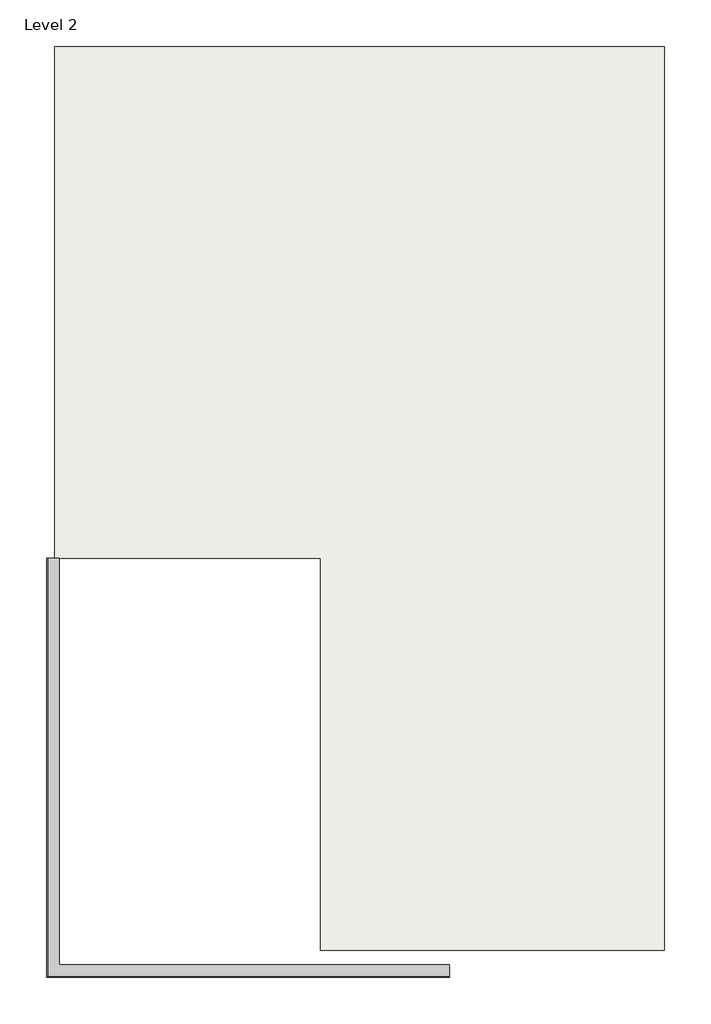
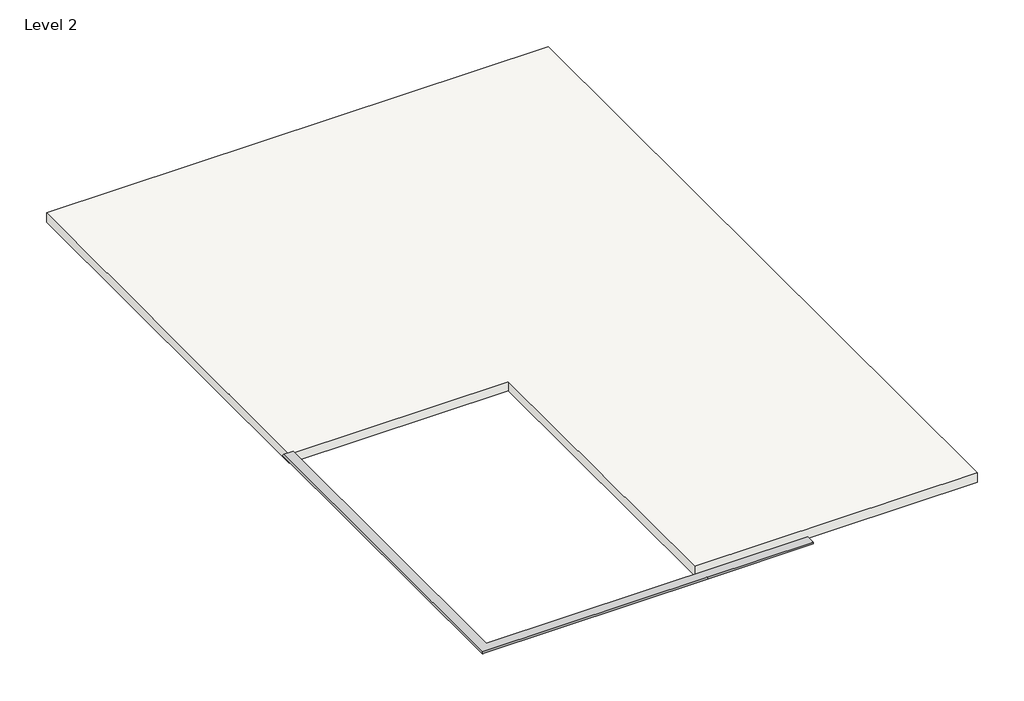
# One storey: 1 proxy, 1 roof.
"""IFC4 building model written with IfcOpenShell, lengths in millimetres."""

from ifc_helpers import new_model, si_unit, frame, origin, place, context, project, spatial, polyline, outline, extrude, transform, mapped, element, save
from components import generic_models_3_generic_models_3_cf0a2ed0

model = new_model("IFC4")

# Units and contexts
model_context = context("Model", 3, world=origin())
ifc_project = project(units=[si_unit("LENGTHUNIT", "METRE", prefix="MILLI")], contexts=[model_context])

# Site, building, storey
site = spatial("IfcSite", under=ifc_project)
building = spatial("IfcBuilding", under=site)
storey = spatial("IfcBuildingStorey", under=building, Name="Level 2", Elevation=6705.6)

# Proxy
placement = place(None, origin())
generic_models_3_generic_models_3_shape = generic_models_3_generic_models_3_cf0a2ed0(model_context)
element("IfcBuildingElementProxy", 1, Name="Generic Models 3 : Generic Models 3", ObjectType="Generic Models 3 : Generic Models 3", at=placement, inside=storey, context=model_context, shape_type="MappedRepresentation", body=[
    mapped(generic_models_3_generic_models_3_shape, transform((0.0, 0.0, 0.0), x_axis=(1.0, 0.0, 0.0), y_axis=(0.0, 1.0, 0.0), z_axis=(0.0, 0.0, 1.0))),
])

# Roof
element("IfcRoof", 2, ObjectType="6\"", at=placement, inside=storey, context=model_context, shape_type="SweptSolid", body=[
    extrude(outline(polyline([(-7937.8525595, 8209.9132107), (-165.4525595, 8209.9132107), (-165.4525595, -3296.2867893), (-4546.9525595, -3296.2867893), (-4546.9525595, 1694.8132107), (-7937.8525595, 1694.8132107), (-7937.8525595, 8209.9132107)])), frame((0.0, 0.0, 6705.6), z_axis=(0.0, 0.0, 1.0), x_axis=(1.0, 0.0, 0.0)), (0.0, 0.0, 1.0), 152.4),
])

save(model, "model.ifc")

# Revit data of these elements
# Type "6\""
#   Layers, outside or top first: 152.4 mm "Steel Purlins" (function 1)
# Element 1 (IfcBuildingElementProxy, "Generic Models 3 : Generic Models 3")
#   Phase Created = New Construction
# Element 2 (IfcRoof, "6\"")
#   built-in parameter 1001705 = 22.5 (stored number, unit not read)
#   built-in parameter 1001710 = 33615
#   Phase Created = New Construction
#   Materials on its faces: "Steel Purlins", "Aluminium", "Paint - White Lining"
# Materials
#   "Steel Purlins": class "Metal", colour RGB 247 247 247, transparency 0, Description = "Light gauge steel purlins", Cost = 0
#   "Aluminium": class "Metal", colour RGB 247 247 247, transparency 0, Description = "Aluminium 6061", Cost = 0
#   "Paint - White Lining": class "Paint", colour RGB 239 247 247, transparency 0, Cost = 0
